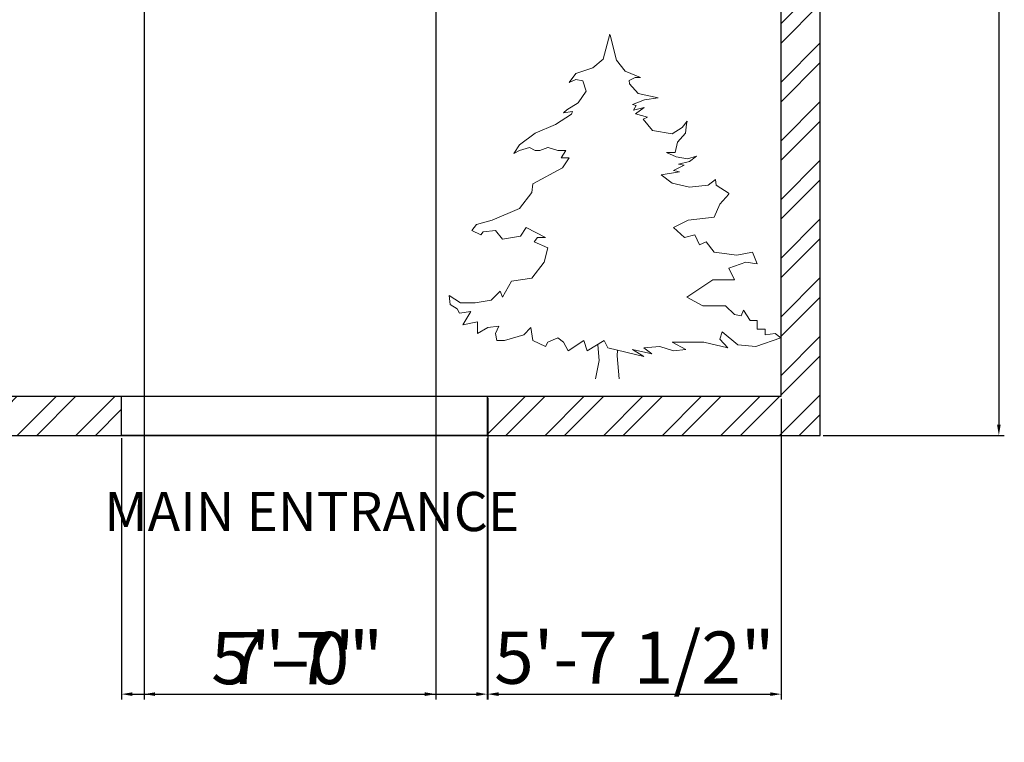
# Model space of a CAD drawing. Units: inches. Extents: x 2588 to 3237, y 2402 to 3178.
# Tile 2 of 4: x 2878 to 3104, y 2402 to 2568. Entities that reach past the tile are written whole.
import ezdxf

# ---------------------------------------------------------------- set-up
doc = ezdxf.new("R2010")
doc.units = ezdxf.units.IN
for name, color, linetype, lineweight in [('A-ANNO-DIMS', 2, 'Continuous', 18), ('A-ANNO-TEXT', 7, 'Continuous', 18), ('L-GATE', 4, 'Continuous', 25), ('L-PLNT-TREE', 3, 'Continuous', 18), ('L-WALL', 7, 'Continuous', 30), ('L-WALL-PATT', 252, 'Continuous', 13)]:
    doc.layers.add(name, color=color, linetype=linetype, lineweight=lineweight)
doc.styles.get("Standard").update_dxf_attribs({"font": 'arial.ttf'})
doc.dimstyles.new('ISO-25', dxfattribs={"dimtxt": 12, "dimasz": 2.5, "dimexe": 1.25, "dimexo": 0.625, "dimtad": 1, "dimdec": 1, "dimlunit": 4, "dimtxsty": 'Standard', "dimcen": 2.5, "dimadec": 0, "dimazin": 0, "dimtfac": 1, "dimtdec": 1, "dimtmove": 0, "dimatfit": 3, "dimfxl": 1, "dimarcsym": 0})

# ---------------------------------------------------------------- blocks, each defined once
blk = doc.blocks.new('*U19')
for p, q in [((-8.263, 7.598), (-8.747, 14.105)), ((-0.771, 9.56), (-0.69, 11.833)), ((0, 0), (-0.771, 9.56)), ((-9.75, 0), (-8.263, 7.598))]:
    blk.add_line(p, q)
for points in [[(-3.9, 142.35), (-6.596, 132.037), (-10.801, 128.443), (-17.81, 126.047), (-20.614, 122.452), (-17.81, 123.65), (-15.007, 123.051), (-13.605, 118.858), (-16.876, 114.065), (-21.549, 111.07), (-22.951, 109.872), (-19.212, 110.471), (-19.68, 109.273), (-26.222, 105.079), (-34.633, 101.485), (-41.175, 96.693), (-43.511, 93.098), (-41.175, 94.296), (-36.969, 95.494), (-34.633, 94.296), (-32.764, 94.296), (-29.493, 95.494)], [(-3.759, 141.97), (-1.074, 131.643), (2.437, 127.141), (8.84, 124.493), (6.568, 124.493), (4.09, 123.169), (4.296, 121.846), (7.807, 117.874), (16.069, 116.02), (10.492, 115.226), (5.535, 113.372), (6.981, 112.843), (5.948, 110.989), (10.286, 112.048), (6.775, 109.401), (11.732, 108.077), (9.873, 107.282), (13.797, 102.516), (21.852, 101.192), (25.983, 103.84), (28.048, 106.488), (27.842, 105.164), (27.429, 101.457), (24.124, 97.75), (23.091, 93.513), (19.58, 93.513), (23.505, 91.66), (28.255, 90.866), (31.973, 91.925), (29.081, 89.806), (24.537, 88.747), (26.809, 88.218), (22.472, 86.099), (24.95, 85.57), (17.308, 84.246), (21.852, 80.804), (29.081, 79.215), (36.723, 80.009), (39.821, 82.392), (40.028, 80.009), (45.398, 76.567)], [(-29.25, 95.55), (-25.287, 94.296), (-22.016, 94.296), (-23.885, 91.301), (-20.614, 91.301), (-23.418, 87.108), (-35.567, 80.518), (-36.035, 76.924), (-41.175, 70.334), (-52.389, 65.542), (-58.931, 63.744), (-60.8, 61.348), (-57.062, 59.551), (-56.128, 60.749), (-50.987, 61.348), (-48.184, 57.754), (-40.707, 58.952), (-38.371, 62.546), (-30.427, 58.353), (-33.698, 58.353), (-35.1, 56.556), (-29.493, 54.159), (-30.894, 48.169), (-36.035, 41.579), (-44.446, 40.381), (-48.184, 33.791), (-49.118, 36.188), (-52.857, 32.593), (-59.399, 31.395), (-65.473, 31.395), (-70.146, 34.39), (-69.679, 30.796), (-66.875, 28.999), (-65.941, 27.202), (-61.268, 27.801), (-64.539, 22.409), (-58.464, 23.607), (-58.464, 18.815), (-54.258, 21.211), (-49.586, 21.81), (-50.987, 18.815), (-50.52, 15.82), (-47.249, 15.82), (-39.306, 18.216), (-36.502, 21.211), (-35.567, 15.82), (-30.427, 13.423), (-29.493, 15.221), (-25.287, 17.018), (-22.951, 15.221), (-21.081, 11.626), (-14.539, 15.82), (-13.138, 11.626), (-6.128, 15.82), (-4.726, 12.824), (10.226, 9.23), (5.554, 12.225), (13.497, 10.428), (10.226, 12.824), (16.768, 13.423), (22.376, 11.626), (27.516, 12.225), (21.909, 15.221), (34.993, 15.221), (44.806, 12.824), (41.535, 16.419), (42.469, 19.414), (49.011, 14.023), (56.487, 13.423), (66.768, 17.018), (64.431, 18.815), (60.226, 18.216), (60.226, 20.612), (56.955, 20.612), (56.955, 24.206), (54.151, 24.206), (51.348, 28.4), (50.413, 26.004), (47.609, 26.603), (43.871, 30.197), (38.731, 30.197), (34.525, 30.197), (27.983, 33.791), (38.731, 40.98), (47.609, 40.98), (45.273, 45.773), (52.282, 48.169), (56.955, 47.57), (55.086, 52.362), (48.544, 51.164), (39.198, 52.362), (35.927, 56.556), (33.123, 55.357), (31.254, 59.551), (27.049, 58.353), (22.376, 62.546), (28.451, 65.542), (39.198, 66.74), (41.535, 72.131), (45.273, 76.325)]]:
    blk.add_lwpolyline(points)
blk = doc.blocks.new('*D23')
at = {"layer": 'A-ANNO-DIMS', "color": 0, "lineweight": -2, "transparency": 16777216}
for p, q in [((3062.02, 3030.83), (3103.65, 3030.83)), ((3102.4, 3028.33), (3102.4, 2475.33)), ((3062.02, 2472.83), (3103.65, 2472.83))]:
    blk.add_line(p, q, dxfattribs=at)
at = {"layer": 'A-ANNO-DIMS', "color": 0, "transparency": 16777216}
for points in [[(3101.99, 3028.33), (3102.82, 3028.33), (3102.4, 3030.83)], [(3101.99, 2475.33), (3102.82, 2475.33), (3102.4, 2472.83)]]:
    blk.add_solid(points, dxfattribs=at)
at = {"layer": 'Defpoints', "color": 0, "transparency": 16777216}
for p in [(3061.4, 3030.83), (3061.4, 2472.83), (3102.4, 2472.83)]:
    blk.add_point(p, dxfattribs=at)
at = {"layer": 'A-ANNO-DIMS', "color": 0, "transparency": 16777216, "insert": (3095.65, 2751.83), "char_height": 12, "attachment_point": 5, "rotation": 90}
blk.add_mtext('46\'-6"', dxfattribs=at)
blk = doc.blocks.new('*D53')
at = {"layer": 'A-ANNO-DIMS', "color": 0, "lineweight": -2, "transparency": 16777216}
for p, q in [((2900.91, 2472.21), (2900.91, 2412.16)), ((2984.91, 2472.21), (2984.91, 2412.16)), ((2903.41, 2413.41), (2982.41, 2413.41))]:
    blk.add_line(p, q, dxfattribs=at)
at = {"layer": 'A-ANNO-DIMS', "color": 0, "transparency": 16777216}
for points in [[(2903.41, 2413.83), (2903.41, 2412.99), (2900.91, 2413.41)], [(2982.41, 2413.83), (2982.41, 2412.99), (2984.91, 2413.41)]]:
    blk.add_solid(points, dxfattribs=at)
at = {"layer": 'Defpoints', "color": 0, "transparency": 16777216}
for p in [(2900.91, 2472.83), (2984.91, 2472.83), (2984.91, 2413.41)]:
    blk.add_point(p, dxfattribs=at)
at = {"layer": 'A-ANNO-DIMS', "color": 0, "transparency": 16777216, "insert": (2942.91, 2420.16), "char_height": 12, "attachment_point": 5}
blk.add_mtext('7\'-0"', dxfattribs=at)
blk = doc.blocks.new('*D54')
at = {"layer": 'A-ANNO-DIMS', "color": 0, "lineweight": -2, "transparency": 16777216}
for p, q in [((2985, 2481.47), (2985, 2412.16)), ((3052.4, 2481.21), (3052.4, 2412.16)), ((2987.5, 2413.41), (3049.9, 2413.41))]:
    blk.add_line(p, q, dxfattribs=at)
at = {"layer": 'A-ANNO-DIMS', "color": 0, "transparency": 16777216}
for points in [[(2987.5, 2413.83), (2987.5, 2412.99), (2985, 2413.41)], [(3049.9, 2413.83), (3049.9, 2412.99), (3052.4, 2413.41)]]:
    blk.add_solid(points, dxfattribs=at)
at = {"layer": 'Defpoints', "color": 0, "transparency": 16777216}
for p in [(2985, 2482.09), (3052.4, 2481.83), (3052.4, 2413.41)]:
    blk.add_point(p, dxfattribs=at)
at = {"layer": 'A-ANNO-DIMS', "color": 0, "transparency": 16777216, "insert": (3018.7, 2420.24), "char_height": 12, "attachment_point": 5}
blk.add_mtext('5\'-7 1/2"', dxfattribs=at)
blk = doc.blocks.new('*D57')
at = {"layer": 'A-ANNO-DIMS', "color": 0, "lineweight": -2, "transparency": 16777216}
for p, q in [((2906.11, 2875.21), (2906.11, 2412.16)), ((2973.06, 2875.21), (2973.06, 2412.16)), ((2908.61, 2413.41), (2970.56, 2413.41))]:
    blk.add_line(p, q, dxfattribs=at)
at = {"layer": 'A-ANNO-DIMS', "color": 0, "transparency": 16777216}
for points in [[(2908.61, 2413.83), (2908.61, 2412.99), (2906.11, 2413.41)], [(2970.56, 2413.83), (2970.56, 2412.99), (2973.06, 2413.41)]]:
    blk.add_solid(points, dxfattribs=at)
at = {"layer": 'Defpoints', "color": 0, "transparency": 16777216}
for p in [(2906.11, 2875.83), (2973.06, 2875.83), (2973.06, 2413.41)]:
    blk.add_point(p, dxfattribs=at)
at = {"layer": 'A-ANNO-DIMS', "color": 0, "transparency": 16777216, "insert": (2939.58, 2420.14), "char_height": 12, "attachment_point": 5}
blk.add_mtext('5\'-7"', dxfattribs=at)

msp = doc.modelspace()

# ---------------------------------------------------------------- hatches: boundary and pattern name
at = {"layer": 'L-WALL-PATT'}
h = msp.add_hatch(dxfattribs=at)
h.set_pattern_fill('ANSI32', color=256)
h.paths.add_polyline_path([(3016.4, 2700.26), (3007.4, 2700.26), (3007.4, 2634.83), (2956.08, 2634.83, -0.03766), (2956.42, 2630.33), (2956.42, 2625.83), (3016.4, 2625.83)], flags=17)
h.paths.add_polyline_path([(3061.4, 2985.83), (3061.4, 3021.83), (3061.4, 3030.83), (3052.4, 3030.83), (3016.4, 3030.83), (2716.4, 3030.83), (2680.4, 3030.83), (2671.4, 3030.83), (2671.4, 3021.83), (2671.4, 2985.83), (2671.4, 2625.83), (2671.4, 2481.83), (2671.4, 2472.83), (2680.4, 2472.83), (2716.4, 2472.83), (2836.4, 2472.83), (2900.91, 2472.83), (2900.91, 2481.83), (2836.4, 2481.83), (2716.4, 2481.83), (2680.4, 2481.83), (2680.4, 2625.83), (2680.4, 2985.83), (2680.4, 3021.83), (2716.4, 3021.83), (3016.4, 3021.83), (3052.4, 3021.83), (3052.4, 2985.83), (3052.4, 2625.83), (3052.4, 2481.83), (2984.91, 2481.83), (2984.91, 2472.83), (3052.4, 2472.83), (3061.4, 2472.83), (3061.4, 2481.83), (3061.4, 2625.83)])

# ---------------------------------------------------------------- linework, layer by layer
at = {"layer": 'L-GATE'}
msp.add_lwpolyline([(2900.91, 2481.83), (2984.91, 2481.83), (2984.91, 2472.83), (2900.91, 2472.83)], close=True, dxfattribs=at)
at = {"layer": 'L-WALL'}
for p, q in [((3052.4, 2481.83), (3052.4, 2625.83)), ((3061.4, 2481.83), (3061.4, 2625.83)), ((2836.4, 2481.83), (3052.4, 2481.83)), ((3061.4, 2472.83), (3061.4, 2481.83)), ((2836.4, 2472.83), (3052.4, 2472.83)), ((3052.4, 2472.83), (3061.4, 2472.83))]:
    msp.add_line(p, q, dxfattribs=at)

# ---------------------------------------------------------------- block references
at = {"layer": 'L-PLNT-TREE', "xscale": 0.5564142683531474, "yscale": 0.5564142683531474, "zscale": 0.5564142683531474}
msp.add_blockref('*U19', (3015.19, 2485.81), dxfattribs=at)

# ---------------------------------------------------------------- texts
at = {"layer": 'A-ANNO-TEXT'}
msp.add_text('MAIN ENTRANCE', height=9, dxfattribs=at).set_placement((2896.94, 2450.86))

# ---------------------------------------------------------------- dimensions: what is measured, and where the dimension line sits
at = {"layer": 'A-ANNO-DIMS'}
dim = msp.add_linear_dim(base=(3102.4, 2472.83), p1=(3061.4, 3030.83), p2=(3061.4, 2472.83), angle=90, dimstyle='ISO-25', override={"dimclrd": 0, "dimclre": 0, "dimclrt": 0}, dxfattribs=at)
dim.commit()
dim.dimension.update_dxf_attribs({"geometry": '*D23', "text_midpoint": (3095.65, 2751.83)})
for base, p1, p2, picture, middle in [((2973.0581, 2413.4091), (2906.1054, 2875.8331), (2973.0581, 2875.8331), '*D57', (2939.5817, 2420.1364)), ((3052.4, 2413.41), (2985, 2482.09), (3052.4, 2481.83), '*D54', (3018.7, 2420.24)), ((2984.91, 2413.41), (2900.91, 2472.83), (2984.91, 2472.83), '*D53', (2942.91, 2420.16))]:
    dim = msp.add_linear_dim(base=base, p1=p1, p2=p2, dimstyle='ISO-25', override={"dimdec": 1, "dimlfac": 1, "dimrnd": 0, "dimzin": 1, "dimdsep": 46, "dimlunit": 4, "dimfrac": 2}, dxfattribs=at)
    dim.commit()
    dim.dimension.update_dxf_attribs({"geometry": picture, "text_midpoint": middle})

doc.saveas('drawing.dxf')
